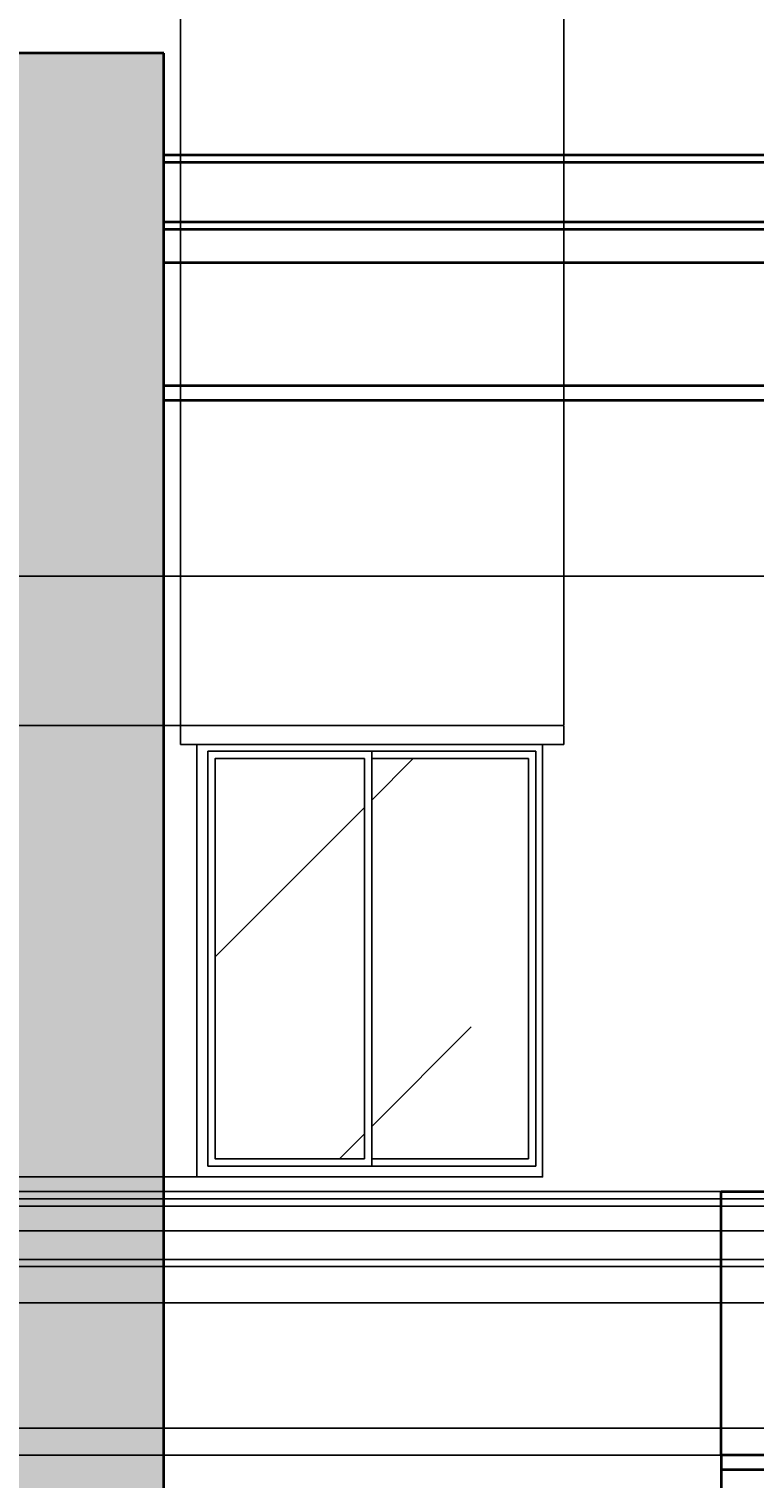
# Model space of a CAD drawing. Units: inches. Extents: x 93 to 565, y 123 to 656.
# Tile 7 of 18: x 192 to 291, y 324 to 522. Entities that reach past the tile are written whole.
import ezdxf

# ---------------------------------------------------------------- set-up
doc = ezdxf.new("R2010")
doc.units = ezdxf.units.IN
doc.header["$MEASUREMENT"] = 0
for name, color, linetype, lineweight in [('A-ANNO-DIMS', 2, 'Continuous', 18), ('A-ELEV', 7, 'Continuous', 35), ('A-GLAZ', 4, 'Continuous', 25), ('A-WALL-PATT', 8, 'Continuous', 13)]:
    doc.layers.add(name, color=color, linetype=linetype, lineweight=lineweight)
doc.styles.get("Standard").update_dxf_attribs({"font": 'arial.ttf'})
doc.dimstyles.get("Standard").update_dxf_attribs({"dimtxt": 0.18, "dimasz": 0.18, "dimexe": 0.18, "dimexo": 0.0625, "dimgap": 0.09, "dimtad": 0, "dimtih": 1, "dimtoh": 1, "dimdec": 4, "dimzin": 0, "dimdsep": 46, "dimtxsty": 'Standard', "dimcen": 0.09, "dimadec": 0, "dimazin": 0, "dimtfac": 1, "dimtdec": 4, "dimtofl": 0, "dimtmove": 0, "dimatfit": 3, "dimfxl": 1, "dimtolj": 1, "dimtzin": 0, "dimarcsym": 0})

# ---------------------------------------------------------------- blocks, each defined once
blk = doc.blocks.new('*U6')
for p, q in [((38.1, 38.1), (38.1, 1476.3)), ((38.1, 1476.3), (607.2, 1476.3)), ((607.2, 38.1), (607.2, 1476.3)), ((607.2, 1476.3), (1176.3, 1476.3)), ((1176.3, 1476.3), (1176.3, 38.1)), ((607.2, 38.1), (38.1, 38.1)), ((1176.3, 38.1), (607.2, 38.1))]:
    blk.add_line(p, q)
blk.add_lwpolyline([(0, 0), (1200, 0), (1200, 1500), (0, 1500)], close=True)
for points in [[(581.8, 1450.9), (581.8, 63.5), (63.5, 63.5), (63.5, 1450.9), (581.8, 1450.9)], [(607.2, 1450.9), (1150.9, 1450.9), (1150.9, 63.5), (607.2, 63.5)]]:
    blk.add_lwpolyline(points)
blk = doc.blocks.new('*D26')
at = {"layer": 'A-ANNO-DIMS', "color": 0, "lineweight": -2, "transparency": 16777216}
for p, q in [((119.08, 519.16), (119.08, 656.13)), ((119.26, 655.95), (328.79, 655.95)), ((538.9, 655.95), (329.37, 655.95)), ((539.08, 630.47), (539.08, 656.13))]:
    blk.add_line(p, q, dxfattribs=at)
at = {"layer": 'A-ANNO-DIMS', "color": 0, "transparency": 16777216}
for points in [[(119.26, 655.98), (119.26, 655.92), (119.08, 655.95)], [(538.9, 655.98), (538.9, 655.92), (539.08, 655.95)]]:
    blk.add_solid(points, dxfattribs=at)
at = {"layer": 'Defpoints', "color": 0, "transparency": 16777216}
for p in [(539.08, 655.95), (539.08, 630.4), (119.08, 519.1)]:
    blk.add_point(p, dxfattribs=at)
at = {"layer": 'A-ANNO-DIMS', "color": 0, "transparency": 16777216, "insert": (329.08, 655.95), "char_height": 0.18, "attachment_point": 5}
blk.add_mtext('\\A1;420', dxfattribs=at)
blk = doc.blocks.new('*D27')
at = {"layer": 'A-ANNO-DIMS', "color": 0, "lineweight": -2, "transparency": 16777216}
for p, q in [((210.54, 519.04), (210.54, 134)), ((119.08, 159.67), (119.08, 134)), ((119.26, 134.18), (164.42, 134.18)), ((210.36, 134.18), (165.21, 134.18))]:
    blk.add_line(p, q, dxfattribs=at)
at = {"layer": 'A-ANNO-DIMS', "color": 0, "transparency": 16777216}
for points in [[(119.26, 134.21), (119.26, 134.15), (119.08, 134.18)], [(210.36, 134.21), (210.36, 134.15), (210.54, 134.18)]]:
    blk.add_solid(points, dxfattribs=at)
at = {"layer": 'Defpoints', "color": 0, "transparency": 16777216}
for p in [(210.54, 519.1), (119.08, 159.73), (210.54, 134.18)]:
    blk.add_point(p, dxfattribs=at)
at = {"layer": 'A-ANNO-DIMS', "color": 0, "transparency": 16777216, "insert": (164.81, 134.18), "char_height": 0.18, "attachment_point": 5}
blk.add_mtext('\\A1;91.46', dxfattribs=at)
blk = doc.blocks.new('*D28')
at = {"layer": 'A-ANNO-DIMS', "color": 0, "lineweight": -2, "transparency": 16777216}
for p, q in [((210.54, 519.04), (210.54, 134)), ((295.69, 183.67), (295.69, 134)), ((210.72, 134.18), (252.72, 134.18)), ((295.51, 134.18), (253.51, 134.18))]:
    blk.add_line(p, q, dxfattribs=at)
at = {"layer": 'A-ANNO-DIMS', "color": 0, "transparency": 16777216}
for points in [[(210.72, 134.21), (210.72, 134.15), (210.54, 134.18)], [(295.51, 134.21), (295.51, 134.15), (295.69, 134.18)]]:
    blk.add_solid(points, dxfattribs=at)
at = {"layer": 'Defpoints', "color": 0, "transparency": 16777216}
for p in [(210.54, 519.1), (295.69, 183.73), (295.69, 134.18)]:
    blk.add_point(p, dxfattribs=at)
at = {"layer": 'A-ANNO-DIMS', "color": 0, "transparency": 16777216, "insert": (253.12, 134.18), "char_height": 0.18, "attachment_point": 5}
blk.add_mtext('\\A1;85.14', dxfattribs=at)
blk = doc.blocks.new('*D31')
at = {"layer": 'A-ANNO-DIMS', "color": 0, "lineweight": -2, "transparency": 16777216}
for p, q in [((417.87, 630.4), (564.81, 630.4)), ((564.63, 630.22), (564.63, 395.25)), ((564.63, 159.91), (564.63, 394.89)), ((119.14, 159.73), (564.81, 159.73))]:
    blk.add_line(p, q, dxfattribs=at)
at = {"layer": 'A-ANNO-DIMS', "color": 0, "transparency": 16777216}
for points in [[(564.6, 630.22), (564.66, 630.22), (564.63, 630.4)], [(564.6, 159.91), (564.66, 159.91), (564.63, 159.73)]]:
    blk.add_solid(points, dxfattribs=at)
at = {"layer": 'Defpoints', "color": 0, "transparency": 16777216}
for p in [(417.81, 630.4), (564.63, 630.4), (119.08, 159.73)]:
    blk.add_point(p, dxfattribs=at)
at = {"layer": 'A-ANNO-DIMS', "color": 0, "transparency": 16777216, "insert": (564.63, 395.07), "char_height": 0.18, "attachment_point": 5}
blk.add_mtext('\\A1;470.7', dxfattribs=at)
blk = doc.blocks.new('*D34')
at = {"layer": 'A-ANNO-DIMS', "color": 0, "lineweight": -2, "transparency": 16777216}
for p, q in [((286.62, 363.73), (93.35, 363.73)), ((93.53, 363.55), (93.53, 338.52)), ((93.53, 313.13), (93.53, 338.16)), ((286.62, 312.95), (93.35, 312.95))]:
    blk.add_line(p, q, dxfattribs=at)
at = {"layer": 'A-ANNO-DIMS', "color": 0, "transparency": 16777216}
for points in [[(93.5, 363.55), (93.56, 363.55), (93.53, 363.73)], [(93.5, 313.13), (93.56, 313.13), (93.53, 312.95)]]:
    blk.add_solid(points, dxfattribs=at)
at = {"layer": 'Defpoints', "color": 0, "transparency": 16777216}
for p in [(93.53, 363.73), (286.69, 363.73), (286.69, 312.95)]:
    blk.add_point(p, dxfattribs=at)
at = {"layer": 'A-ANNO-DIMS', "color": 0, "transparency": 16777216, "insert": (93.53, 338.34), "char_height": 0.18, "attachment_point": 5}
blk.add_mtext('\\A1;50.78', dxfattribs=at)
blk = doc.blocks.new('*D35')
at = {"layer": 'A-ANNO-DIMS', "color": 0, "lineweight": -2, "transparency": 16777216}
for p, q in [((119.02, 519.1), (93.35, 519.1)), ((93.53, 518.92), (93.53, 441.6)), ((93.53, 363.91), (93.53, 441.23)), ((286.62, 363.73), (93.35, 363.73))]:
    blk.add_line(p, q, dxfattribs=at)
at = {"layer": 'A-ANNO-DIMS', "color": 0, "transparency": 16777216}
for points in [[(93.5, 518.92), (93.56, 518.92), (93.53, 519.1)], [(93.5, 363.91), (93.56, 363.91), (93.53, 363.73)]]:
    blk.add_solid(points, dxfattribs=at)
at = {"layer": 'Defpoints', "color": 0, "transparency": 16777216}
for p in [(93.53, 519.1), (119.08, 519.1), (286.69, 363.73)]:
    blk.add_point(p, dxfattribs=at)
at = {"layer": 'A-ANNO-DIMS', "color": 0, "transparency": 16777216, "insert": (93.53, 441.42), "char_height": 0.18, "attachment_point": 5}
blk.add_mtext('\\A1;155.37', dxfattribs=at)
blk = doc.blocks.new('*D36')
at = {"layer": 'A-ANNO-DIMS', "color": 0, "lineweight": -2, "transparency": 16777216}
for p, q in [((417.75, 594.4), (93.35, 594.4)), ((93.53, 594.22), (93.53, 556.93)), ((93.53, 519.28), (93.53, 556.57)), ((119.02, 519.1), (93.35, 519.1))]:
    blk.add_line(p, q, dxfattribs=at)
at = {"layer": 'A-ANNO-DIMS', "color": 0, "transparency": 16777216}
for points in [[(93.5, 594.22), (93.56, 594.22), (93.53, 594.4)], [(93.5, 519.28), (93.56, 519.28), (93.53, 519.1)]]:
    blk.add_solid(points, dxfattribs=at)
at = {"layer": 'Defpoints', "color": 0, "transparency": 16777216}
for p in [(93.53, 594.4), (417.81, 594.4), (119.08, 519.1)]:
    blk.add_point(p, dxfattribs=at)
at = {"layer": 'A-ANNO-DIMS', "color": 0, "transparency": 16777216, "insert": (93.53, 556.75), "char_height": 0.18, "attachment_point": 5}
blk.add_mtext('\\A1;75.3', dxfattribs=at)
blk = doc.blocks.new('*D64')
at = {"layer": 'A-ANNO-DIMS', "color": 0, "lineweight": -2, "transparency": 16777216}
for p, q in [((212.83, 427.41), (212.83, 656.13)), ((213.01, 655.95), (238.63, 655.95)), ((265.03, 655.95), (239.41, 655.95)), ((265.21, 427.41), (265.21, 656.13))]:
    blk.add_line(p, q, dxfattribs=at)
at = {"layer": 'A-ANNO-DIMS', "color": 0, "transparency": 16777216}
for points in [[(213.01, 655.98), (213.01, 655.92), (212.83, 655.95)], [(265.03, 655.98), (265.03, 655.92), (265.21, 655.95)]]:
    blk.add_solid(points, dxfattribs=at)
at = {"layer": 'Defpoints', "color": 0, "transparency": 16777216}
for p in [(265.21, 655.95), (212.83, 427.35), (265.21, 427.35)]:
    blk.add_point(p, dxfattribs=at)
at = {"layer": 'A-ANNO-DIMS', "color": 0, "transparency": 16777216, "insert": (239.02, 655.95), "char_height": 0.18, "attachment_point": 5}
blk.add_mtext('\\A1;52.39', dxfattribs=at)
blk = doc.blocks.new('*D65')
at = {"layer": 'A-ANNO-DIMS', "color": 0, "lineweight": -2, "transparency": 16777216}
for p, q in [((265.15, 427.35), (93.35, 427.35)), ((93.53, 427.17), (93.53, 396.71)), ((93.53, 365.89), (93.53, 396.35)), ((262.24, 365.71), (93.35, 365.71))]:
    blk.add_line(p, q, dxfattribs=at)
at = {"layer": 'A-ANNO-DIMS', "color": 0, "transparency": 16777216}
for points in [[(93.5, 427.17), (93.56, 427.17), (93.53, 427.35)], [(93.5, 365.89), (93.56, 365.89), (93.53, 365.71)]]:
    blk.add_solid(points, dxfattribs=at)
at = {"layer": 'Defpoints', "color": 0, "transparency": 16777216}
for p in [(93.53, 427.35), (265.21, 427.35), (262.3, 365.71)]:
    blk.add_point(p, dxfattribs=at)
at = {"layer": 'A-ANNO-DIMS', "color": 0, "transparency": 16777216, "insert": (93.53, 396.53), "char_height": 0.18, "attachment_point": 5}
blk.add_mtext('\\A1;61.64', dxfattribs=at)
blk = doc.blocks.new('*D72')
at = {"layer": 'A-ANNO-DIMS', "color": 0, "lineweight": -2, "transparency": 16777216}
for p, q in [((295.62, 447.73), (93.35, 447.73)), ((93.53, 447.55), (93.53, 405.91)), ((93.53, 363.91), (93.53, 405.55)), ((286.62, 363.73), (93.35, 363.73))]:
    blk.add_line(p, q, dxfattribs=at)
at = {"layer": 'A-ANNO-DIMS', "color": 0, "transparency": 16777216}
for points in [[(93.5, 447.55), (93.56, 447.55), (93.53, 447.73)], [(93.5, 363.91), (93.56, 363.91), (93.53, 363.73)]]:
    blk.add_solid(points, dxfattribs=at)
at = {"layer": 'Defpoints', "color": 0, "transparency": 16777216}
for p in [(295.69, 447.73), (93.53, 363.73), (286.69, 363.73)]:
    blk.add_point(p, dxfattribs=at)
at = {"layer": 'A-ANNO-DIMS', "color": 0, "transparency": 16777216, "insert": (93.53, 405.73), "char_height": 0.18, "attachment_point": 5}
blk.add_mtext('\\A1;84', dxfattribs=at)
blk = doc.blocks.new('*D105')
at = {"layer": 'A-ANNO-DIMS', "color": 0, "lineweight": -2, "transparency": 16777216}
for p, q in [((119.08, 519.16), (119.08, 656.13)), ((119.26, 655.95), (328.54, 655.95)), ((538.9, 655.95), (329.62, 655.95)), ((539.08, 630.47), (539.08, 656.13))]:
    blk.add_line(p, q, dxfattribs=at)
at = {"layer": 'A-ANNO-DIMS', "color": 0, "transparency": 16777216}
for points in [[(119.26, 655.98), (119.26, 655.92), (119.08, 655.95)], [(538.9, 655.98), (538.9, 655.92), (539.08, 655.95)]]:
    blk.add_solid(points, dxfattribs=at)
at = {"layer": 'Defpoints', "color": 0, "transparency": 16777216}
for p in [(539.08, 655.95), (539.08, 630.4), (119.08, 519.1)]:
    blk.add_point(p, dxfattribs=at)
at = {"layer": 'A-ANNO-DIMS', "color": 0, "transparency": 16777216, "insert": (329.08, 655.95), "char_height": 0.18, "attachment_point": 5}
blk.add_mtext('\\A1;420.000', dxfattribs=at)
blk = doc.blocks.new('*D106')
at = {"layer": 'A-ANNO-DIMS', "color": 0, "lineweight": -2, "transparency": 16777216}
for p, q in [((210.54, 519.04), (210.54, 134)), ((119.08, 159.67), (119.08, 134)), ((119.26, 134.18), (164.35, 134.18)), ((210.36, 134.18), (165.28, 134.18))]:
    blk.add_line(p, q, dxfattribs=at)
at = {"layer": 'A-ANNO-DIMS', "color": 0, "transparency": 16777216}
for points in [[(119.26, 134.21), (119.26, 134.15), (119.08, 134.18)], [(210.36, 134.21), (210.36, 134.15), (210.54, 134.18)]]:
    blk.add_solid(points, dxfattribs=at)
at = {"layer": 'Defpoints', "color": 0, "transparency": 16777216}
for p in [(210.54, 519.1), (119.08, 159.73), (210.54, 134.18)]:
    blk.add_point(p, dxfattribs=at)
at = {"layer": 'A-ANNO-DIMS', "color": 0, "transparency": 16777216, "insert": (164.81, 134.18), "char_height": 0.18, "attachment_point": 5}
blk.add_mtext('\\A1;91.465', dxfattribs=at)
blk = doc.blocks.new('*D107')
at = {"layer": 'A-ANNO-DIMS', "color": 0, "lineweight": -2, "transparency": 16777216}
for p, q in [((210.54, 519.04), (210.54, 134)), ((295.69, 183.67), (295.69, 134)), ((210.72, 134.18), (252.65, 134.18)), ((295.51, 134.18), (253.58, 134.18))]:
    blk.add_line(p, q, dxfattribs=at)
at = {"layer": 'A-ANNO-DIMS', "color": 0, "transparency": 16777216}
for points in [[(210.72, 134.21), (210.72, 134.15), (210.54, 134.18)], [(295.51, 134.21), (295.51, 134.15), (295.69, 134.18)]]:
    blk.add_solid(points, dxfattribs=at)
at = {"layer": 'Defpoints', "color": 0, "transparency": 16777216}
for p in [(210.54, 519.1), (295.69, 183.73), (295.69, 134.18)]:
    blk.add_point(p, dxfattribs=at)
at = {"layer": 'A-ANNO-DIMS', "color": 0, "transparency": 16777216, "insert": (253.12, 134.18), "char_height": 0.18, "attachment_point": 5}
blk.add_mtext('\\A1;85.143', dxfattribs=at)
blk = doc.blocks.new('*D110')
at = {"layer": 'A-ANNO-DIMS', "color": 0, "lineweight": -2, "transparency": 16777216}
for p, q in [((417.87, 630.4), (564.81, 630.4)), ((564.63, 630.22), (564.63, 395.25)), ((564.63, 159.91), (564.63, 394.89)), ((119.14, 159.73), (564.81, 159.73))]:
    blk.add_line(p, q, dxfattribs=at)
at = {"layer": 'A-ANNO-DIMS', "color": 0, "transparency": 16777216}
for points in [[(564.6, 630.22), (564.66, 630.22), (564.63, 630.4)], [(564.6, 159.91), (564.66, 159.91), (564.63, 159.73)]]:
    blk.add_solid(points, dxfattribs=at)
at = {"layer": 'Defpoints', "color": 0, "transparency": 16777216}
for p in [(417.81, 630.4), (564.63, 630.4), (119.08, 159.73)]:
    blk.add_point(p, dxfattribs=at)
at = {"layer": 'A-ANNO-DIMS', "color": 0, "transparency": 16777216, "insert": (564.63, 395.07), "char_height": 0.18, "attachment_point": 5}
blk.add_mtext('\\A1;470.673', dxfattribs=at)
blk = doc.blocks.new('*D113')
at = {"layer": 'A-ANNO-DIMS', "color": 0, "lineweight": -2, "transparency": 16777216}
for p, q in [((286.62, 363.73), (93.35, 363.73)), ((93.53, 363.55), (93.53, 338.52)), ((93.53, 313.13), (93.53, 338.16)), ((286.62, 312.95), (93.35, 312.95))]:
    blk.add_line(p, q, dxfattribs=at)
at = {"layer": 'A-ANNO-DIMS', "color": 0, "transparency": 16777216}
for points in [[(93.5, 363.55), (93.56, 363.55), (93.53, 363.73)], [(93.5, 313.13), (93.56, 313.13), (93.53, 312.95)]]:
    blk.add_solid(points, dxfattribs=at)
at = {"layer": 'Defpoints', "color": 0, "transparency": 16777216}
for p in [(93.53, 363.73), (286.69, 363.73), (286.69, 312.95)]:
    blk.add_point(p, dxfattribs=at)
at = {"layer": 'A-ANNO-DIMS', "color": 0, "transparency": 16777216, "insert": (93.53, 338.34), "char_height": 0.18, "attachment_point": 5}
blk.add_mtext('\\A1;50.783', dxfattribs=at)
blk = doc.blocks.new('*D114')
at = {"layer": 'A-ANNO-DIMS', "color": 0, "lineweight": -2, "transparency": 16777216}
for p, q in [((119.02, 519.1), (93.35, 519.1)), ((93.53, 518.92), (93.53, 441.6)), ((93.53, 363.91), (93.53, 441.23)), ((286.62, 363.73), (93.35, 363.73))]:
    blk.add_line(p, q, dxfattribs=at)
at = {"layer": 'A-ANNO-DIMS', "color": 0, "transparency": 16777216}
for points in [[(93.5, 518.92), (93.56, 518.92), (93.53, 519.1)], [(93.5, 363.91), (93.56, 363.91), (93.53, 363.73)]]:
    blk.add_solid(points, dxfattribs=at)
at = {"layer": 'Defpoints', "color": 0, "transparency": 16777216}
for p in [(93.53, 519.1), (119.08, 519.1), (286.69, 363.73)]:
    blk.add_point(p, dxfattribs=at)
at = {"layer": 'A-ANNO-DIMS', "color": 0, "transparency": 16777216, "insert": (93.53, 441.42), "char_height": 0.18, "attachment_point": 5}
blk.add_mtext('\\A1;155.368', dxfattribs=at)
blk = doc.blocks.new('*D115')
at = {"layer": 'A-ANNO-DIMS', "color": 0, "lineweight": -2, "transparency": 16777216}
for p, q in [((417.75, 594.4), (93.35, 594.4)), ((93.53, 594.22), (93.53, 556.93)), ((93.53, 519.28), (93.53, 556.57)), ((119.02, 519.1), (93.35, 519.1))]:
    blk.add_line(p, q, dxfattribs=at)
at = {"layer": 'A-ANNO-DIMS', "color": 0, "transparency": 16777216}
for points in [[(93.5, 594.22), (93.56, 594.22), (93.53, 594.4)], [(93.5, 519.28), (93.56, 519.28), (93.53, 519.1)]]:
    blk.add_solid(points, dxfattribs=at)
at = {"layer": 'Defpoints', "color": 0, "transparency": 16777216}
for p in [(93.53, 594.4), (417.81, 594.4), (119.08, 519.1)]:
    blk.add_point(p, dxfattribs=at)
at = {"layer": 'A-ANNO-DIMS', "color": 0, "transparency": 16777216, "insert": (93.53, 556.75), "char_height": 0.18, "attachment_point": 5}
blk.add_mtext('\\A1;75.305', dxfattribs=at)
blk = doc.blocks.new('*D143')
at = {"layer": 'A-ANNO-DIMS', "color": 0, "lineweight": -2, "transparency": 16777216}
for p, q in [((212.83, 427.41), (212.83, 656.13)), ((213.01, 655.95), (238.56, 655.95)), ((265.03, 655.95), (239.48, 655.95)), ((265.21, 427.41), (265.21, 656.13))]:
    blk.add_line(p, q, dxfattribs=at)
at = {"layer": 'A-ANNO-DIMS', "color": 0, "transparency": 16777216}
for points in [[(213.01, 655.98), (213.01, 655.92), (212.83, 655.95)], [(265.03, 655.98), (265.03, 655.92), (265.21, 655.95)]]:
    blk.add_solid(points, dxfattribs=at)
at = {"layer": 'Defpoints', "color": 0, "transparency": 16777216}
for p in [(265.21, 655.95), (212.83, 427.35), (265.21, 427.35)]:
    blk.add_point(p, dxfattribs=at)
at = {"layer": 'A-ANNO-DIMS', "color": 0, "transparency": 16777216, "insert": (239.02, 655.95), "char_height": 0.18, "attachment_point": 5}
blk.add_mtext('\\A1;52.388', dxfattribs=at)
blk = doc.blocks.new('*D144')
at = {"layer": 'A-ANNO-DIMS', "color": 0, "lineweight": -2, "transparency": 16777216}
for p, q in [((265.15, 427.35), (93.35, 427.35)), ((93.53, 427.17), (93.53, 396.71)), ((93.53, 365.89), (93.53, 396.35)), ((262.24, 365.71), (93.35, 365.71))]:
    blk.add_line(p, q, dxfattribs=at)
at = {"layer": 'A-ANNO-DIMS', "color": 0, "transparency": 16777216}
for points in [[(93.5, 427.17), (93.56, 427.17), (93.53, 427.35)], [(93.5, 365.89), (93.56, 365.89), (93.53, 365.71)]]:
    blk.add_solid(points, dxfattribs=at)
at = {"layer": 'Defpoints', "color": 0, "transparency": 16777216}
for p in [(93.53, 427.35), (265.21, 427.35), (262.3, 365.71)]:
    blk.add_point(p, dxfattribs=at)
at = {"layer": 'A-ANNO-DIMS', "color": 0, "transparency": 16777216, "insert": (93.53, 396.53), "char_height": 0.18, "attachment_point": 5}
blk.add_mtext('\\A1;61.638', dxfattribs=at)
blk = doc.blocks.new('*D151')
at = {"layer": 'A-ANNO-DIMS', "color": 0, "lineweight": -2, "transparency": 16777216}
for p, q in [((295.62, 447.73), (93.35, 447.73)), ((93.53, 447.55), (93.53, 405.91)), ((93.53, 363.91), (93.53, 405.55)), ((286.62, 363.73), (93.35, 363.73))]:
    blk.add_line(p, q, dxfattribs=at)
at = {"layer": 'A-ANNO-DIMS', "color": 0, "transparency": 16777216}
for points in [[(93.5, 447.55), (93.56, 447.55), (93.53, 447.73)], [(93.5, 363.91), (93.56, 363.91), (93.53, 363.73)]]:
    blk.add_solid(points, dxfattribs=at)
at = {"layer": 'Defpoints', "color": 0, "transparency": 16777216}
for p in [(295.69, 447.73), (93.53, 363.73), (286.69, 363.73)]:
    blk.add_point(p, dxfattribs=at)
at = {"layer": 'A-ANNO-DIMS', "color": 0, "transparency": 16777216, "insert": (93.53, 405.73), "char_height": 0.18, "attachment_point": 5}
blk.add_mtext('\\A1;84.000', dxfattribs=at)
blk = doc.blocks.new('*D190')
at = {"layer": 'A-ANNO-DIMS', "color": 0, "lineweight": -2, "transparency": 16777216}
for p, q in [((514.58, 348.55), (93.35, 348.55)), ((93.53, 348.37), (93.53, 338.33)), ((93.53, 327.91), (93.53, 337.96)), ((539.02, 327.73), (93.35, 327.73))]:
    blk.add_line(p, q, dxfattribs=at)
at = {"layer": 'A-ANNO-DIMS', "color": 0, "transparency": 16777216}
for points in [[(93.5, 348.37), (93.56, 348.37), (93.53, 348.55)], [(93.5, 327.91), (93.56, 327.91), (93.53, 327.73)]]:
    blk.add_solid(points, dxfattribs=at)
at = {"layer": 'Defpoints', "color": 0, "transparency": 16777216}
for p in [(93.53, 348.55), (514.64, 348.55), (539.08, 327.73)]:
    blk.add_point(p, dxfattribs=at)
at = {"layer": 'A-ANNO-DIMS', "color": 0, "transparency": 16777216, "insert": (93.53, 338.14), "char_height": 0.18, "attachment_point": 5}
blk.add_mtext('\\A1;20.822', dxfattribs=at)
blk = doc.blocks.new('*D191')
at = {"layer": 'A-ANNO-DIMS', "color": 0, "lineweight": -2, "transparency": 16777216}
for p, q in [((514.58, 353.47), (93.35, 353.47)), ((93.53, 353.29), (93.53, 351.2)), ((93.53, 348.73), (93.53, 350.83)), ((514.58, 348.55), (93.35, 348.55))]:
    blk.add_line(p, q, dxfattribs=at)
at = {"layer": 'A-ANNO-DIMS', "color": 0, "transparency": 16777216}
for points in [[(93.5, 353.29), (93.56, 353.29), (93.53, 353.47)], [(93.5, 348.73), (93.56, 348.73), (93.53, 348.55)]]:
    blk.add_solid(points, dxfattribs=at)
at = {"layer": 'Defpoints', "color": 0, "transparency": 16777216}
for p in [(93.53, 353.47), (514.64, 353.47), (514.64, 348.55)]:
    blk.add_point(p, dxfattribs=at)
at = {"layer": 'A-ANNO-DIMS', "color": 0, "transparency": 16777216, "insert": (93.53, 351.01), "char_height": 0.18, "attachment_point": 5}
blk.add_mtext('\\A1;4.918', dxfattribs=at)
blk = doc.blocks.new('*D192')
at = {"layer": 'A-ANNO-DIMS', "color": 0, "lineweight": -2, "transparency": 16777216}
for p, q in [((514.58, 354.47), (93.35, 354.47)), ((514.58, 353.47), (93.35, 353.47)), ((93.53, 354.29), (93.53, 354.15)), ((93.53, 353.65), (93.53, 353.79))]:
    blk.add_line(p, q, dxfattribs=at)
at = {"layer": 'A-ANNO-DIMS', "color": 0, "transparency": 16777216}
for points in [[(93.5, 354.29), (93.56, 354.29), (93.53, 354.47)], [(93.5, 353.65), (93.56, 353.65), (93.53, 353.47)]]:
    blk.add_solid(points, dxfattribs=at)
at = {"layer": 'Defpoints', "color": 0, "transparency": 16777216}
for p in [(93.53, 354.47), (514.64, 354.47), (514.64, 353.47)]:
    blk.add_point(p, dxfattribs=at)
at = {"layer": 'A-ANNO-DIMS', "color": 0, "transparency": 16777216, "insert": (93.53, 353.97), "char_height": 0.18, "attachment_point": 5}
blk.add_mtext('\\A1;1.000', dxfattribs=at)
blk = doc.blocks.new('*D193')
at = {"layer": 'A-ANNO-DIMS', "color": 0, "lineweight": -2, "transparency": 16777216}
for p, q in [((514.58, 358.37), (93.35, 358.37)), ((93.53, 358.19), (93.53, 356.61)), ((514.58, 354.47), (93.35, 354.47)), ((93.53, 354.65), (93.53, 356.24))]:
    blk.add_line(p, q, dxfattribs=at)
at = {"layer": 'A-ANNO-DIMS', "color": 0, "transparency": 16777216}
for points in [[(93.5, 358.19), (93.56, 358.19), (93.53, 358.37)], [(93.5, 354.65), (93.56, 354.65), (93.53, 354.47)]]:
    blk.add_solid(points, dxfattribs=at)
at = {"layer": 'Defpoints', "color": 0, "transparency": 16777216}
for p in [(93.53, 358.37), (514.64, 358.37), (514.64, 354.47)]:
    blk.add_point(p, dxfattribs=at)
at = {"layer": 'A-ANNO-DIMS', "color": 0, "transparency": 16777216, "insert": (93.53, 356.42), "char_height": 0.18, "attachment_point": 5}
blk.add_mtext('\\A1;3.901', dxfattribs=at)
blk = doc.blocks.new('*D194')
at = {"layer": 'A-ANNO-DIMS', "color": 0, "lineweight": -2, "transparency": 16777216}
for p, q in [((524.92, 361.75), (93.35, 361.75)), ((93.53, 361.57), (93.53, 360.24)), ((514.58, 358.37), (93.35, 358.37)), ((93.53, 358.55), (93.53, 359.88))]:
    blk.add_line(p, q, dxfattribs=at)
at = {"layer": 'A-ANNO-DIMS', "color": 0, "transparency": 16777216}
for points in [[(93.5, 361.57), (93.56, 361.57), (93.53, 361.75)], [(93.5, 358.55), (93.56, 358.55), (93.53, 358.37)]]:
    blk.add_solid(points, dxfattribs=at)
at = {"layer": 'Defpoints', "color": 0, "transparency": 16777216}
for p in [(93.53, 361.75), (524.99, 361.75), (514.64, 358.37)]:
    blk.add_point(p, dxfattribs=at)
at = {"layer": 'A-ANNO-DIMS', "color": 0, "transparency": 16777216, "insert": (93.53, 360.06), "char_height": 0.18, "attachment_point": 5}
blk.add_mtext('\\A1;3.374', dxfattribs=at)
blk = doc.blocks.new('*D195')
at = {"layer": 'A-ANNO-DIMS', "color": 0, "lineweight": -2, "transparency": 16777216}
for p, q in [((524.92, 362.75), (93.35, 362.75)), ((93.53, 362.57), (93.53, 362.43)), ((524.92, 361.75), (93.35, 361.75)), ((93.53, 361.93), (93.53, 362.07))]:
    blk.add_line(p, q, dxfattribs=at)
at = {"layer": 'A-ANNO-DIMS', "color": 0, "transparency": 16777216}
for points in [[(93.5, 362.57), (93.56, 362.57), (93.53, 362.75)], [(93.5, 361.93), (93.56, 361.93), (93.53, 361.75)]]:
    blk.add_solid(points, dxfattribs=at)
at = {"layer": 'Defpoints', "color": 0, "transparency": 16777216}
for p in [(93.53, 362.75), (524.99, 362.75), (524.99, 361.75)]:
    blk.add_point(p, dxfattribs=at)
at = {"layer": 'A-ANNO-DIMS', "color": 0, "transparency": 16777216, "insert": (93.53, 362.25), "char_height": 0.18, "attachment_point": 5}
blk.add_mtext('\\A1;1.000', dxfattribs=at)
blk = doc.blocks.new('*D196')
at = {"layer": 'A-ANNO-DIMS', "color": 0, "lineweight": -2, "transparency": 16777216}
for p, q in [((524.92, 363.73), (93.35, 363.73)), ((524.92, 362.75), (93.35, 362.75)), ((93.53, 363.55), (93.53, 363.42)), ((93.53, 362.93), (93.53, 363.06))]:
    blk.add_line(p, q, dxfattribs=at)
at = {"layer": 'A-ANNO-DIMS', "color": 0, "transparency": 16777216}
for points in [[(93.5, 363.55), (93.56, 363.55), (93.53, 363.73)], [(93.5, 362.93), (93.56, 362.93), (93.53, 362.75)]]:
    blk.add_solid(points, dxfattribs=at)
at = {"layer": 'Defpoints', "color": 0, "transparency": 16777216}
for p in [(93.53, 363.73), (524.99, 363.73), (524.99, 362.75)]:
    blk.add_point(p, dxfattribs=at)
at = {"layer": 'A-ANNO-DIMS', "color": 0, "transparency": 16777216, "insert": (93.53, 363.24), "char_height": 0.18, "attachment_point": 5}
blk.add_mtext('\\A1;0.985', dxfattribs=at)
blk = doc.blocks.new('*D198')
at = {"layer": 'A-ANNO-DIMS', "color": 0, "lineweight": -2, "transparency": 16777216}
for p, q in [((515.95, 331.43), (93.35, 331.43)), ((93.53, 331.25), (93.53, 329.76)), ((93.53, 327.91), (93.53, 329.4)), ((539.02, 327.73), (93.35, 327.73))]:
    blk.add_line(p, q, dxfattribs=at)
at = {"layer": 'A-ANNO-DIMS', "color": 0, "transparency": 16777216}
for points in [[(93.5, 331.25), (93.56, 331.25), (93.53, 331.43)], [(93.5, 327.91), (93.56, 327.91), (93.53, 327.73)]]:
    blk.add_solid(points, dxfattribs=at)
at = {"layer": 'Defpoints', "color": 0, "transparency": 16777216}
for p in [(93.53, 331.43), (516.01, 331.43), (539.08, 327.73)]:
    blk.add_point(p, dxfattribs=at)
at = {"layer": 'A-ANNO-DIMS', "color": 0, "transparency": 16777216, "insert": (93.53, 329.58), "char_height": 0.18, "attachment_point": 5}
blk.add_mtext('\\A1;3.701', dxfattribs=at)

msp = doc.modelspace()

# ---------------------------------------------------------------- hatches: boundary and pattern name
at = {"layer": 'A-GLAZ'}
h = msp.add_hatch(dxfattribs=at)
h.set_pattern_fill('GOST_GLASS', color=256, scale=21)
h.set_pattern_definition([(45, (0, 0), (178.19, 0), [105, -147]), (45, (44.55, 0), (178.19, 0), [42, -210]), (45, (0, 44.55), (178.19, 0), [42, -210])])
h.paths.add_polyline_path([(237.9617, 422.832), (217.5562, 422.832), (217.5562, 368.21), (237.9617, 368.21)])
h.paths.add_polyline_path([(260.3673, 422.832), (238.9617, 422.832), (238.9617, 368.21), (260.3673, 368.21)])
at = {"layer": 'A-WALL-PATT'}
h = msp.add_hatch(dxfattribs=at)
h.set_pattern_fill('STARS', color=256, scale=21)
h.paths.add_polyline_path([(210.5443, 507.7323), (210.5443, 519.0999), (119.0794, 519.0999), (119.0794, 507.7323), (119.0794, 183.7323), (210.5443, 183.7323)])
h.paths.add_polyline_path([(187.648, 430.1508), (187.648, 391.4653), (143.2118, 391.4653), (143.2118, 430.1508)], flags=16)
h.paths.add_polyline_path([(187.648, 455.6579), (143.2118, 455.6579), (143.2118, 494.3434), (187.648, 494.3434)], flags=16)
h.paths.add_polyline_path([(184.648, 427.1508), (184.648, 394.4653), (146.2118, 394.4653), (146.2118, 427.1508)], flags=0)
h.paths.add_polyline_path([(184.648, 458.6579), (146.2118, 458.6579), (146.2118, 491.3434), (184.648, 491.3434)], flags=0)
h.paths.add_polyline_path([(187.648, 363.1705), (187.648, 324.485), (143.2118, 324.485), (143.2118, 363.1705)], flags=16)
h.paths.add_polyline_path([(184.648, 360.1705), (184.648, 327.485), (146.2118, 327.485), (146.2118, 360.1705)], flags=0)
h.paths.add_polyline_path([(187.648, 300.3249), (187.648, 261.6394), (143.2118, 261.6394), (143.2118, 300.3249)], flags=16)
h.paths.add_polyline_path([(184.648, 297.3249), (184.648, 264.6394), (146.2118, 264.6394), (146.2118, 297.3249)], flags=0)
h.paths.add_polyline_path([(187.648, 243.6441), (187.648, 204.9587), (143.2118, 204.9587), (143.2118, 243.6441)], flags=16)
h.paths.add_polyline_path([(184.648, 240.6441), (184.648, 207.9587), (146.2118, 207.9587), (146.2118, 240.6441)], flags=0)

# ---------------------------------------------------------------- linework, layer by layer
at = {"layer": 'A-ELEV'}
for p, q in [((210.5443, 519.0999), (119.0794, 519.0999)), ((210.5443, 507.7323), (210.5443, 519.0999)), ((210.5443, 183.7323), (210.5443, 507.7323)), ((399.6946, 505.2018), (210.5443, 505.2018)), ((399.6946, 504.2018), (210.5443, 504.2018)), ((375.0121, 496.0418), (210.5443, 496.0418)), ((375.0121, 495.0418), (210.5443, 495.0418)), ((375.0121, 490.4746), (210.5443, 490.4746)), ((210.5443, 473.7323), (437.1885, 473.7323)), ((210.5443, 471.7323), (437.1885, 471.7323)), ((286.6874, 327.7323), (286.6874, 363.7323)), ((286.6874, 363.7323), (295.6874, 363.7323)), ((295.6874, 327.7323), (286.6874, 327.7323)), ((286.6874, 327.7323), (286.6874, 312.9491)), ((295.6874, 325.7323), (286.6874, 325.7323))]:
    msp.add_line(p, q, dxfattribs=at)
at = {"layer": 'A-GLAZ'}
for p, q in [((265.2145, 427.3478), (212.8266, 427.3478)), ((212.8266, 427.3478), (212.8266, 424.7651)), ((265.2145, 424.7651), (265.2145, 427.3478)), ((212.8266, 424.7651), (216.5562, 424.7651)), ((262.3003, 424.7651), (265.2145, 424.7651))]:
    msp.add_line(p, q, dxfattribs=at)

# ---------------------------------------------------------------- block references
at = {"layer": 'A-GLAZ', "xscale": 0.0393700787401575, "yscale": 0.0393700787401575, "zscale": 0.0393700787401575}
msp.add_blockref('*U6', (215.0562, 365.71), dxfattribs=at)

# ---------------------------------------------------------------- dimensions: what is measured, and where the dimension line sits
at = {"layer": 'A-ANNO-DIMS'}
for base, p1, p2, override, picture, middle in [((539.0794, 655.9548), (119.0794, 519.0999), (539.0794, 630.4048), {"dimdec": 0, "dimlfac": 1, "dimrnd": 0, "dimzin": 0, "dimdsep": 46, "dimlunit": 2}, '*D26', (329.0794, 655.9548)), ((539.0794, 655.9548), (119.0794, 519.0999), (539.0794, 630.4048), {"dimdec": 3, "dimlfac": 1, "dimrnd": 0, "dimzin": 0, "dimdsep": 46, "dimlunit": 2}, '*D105', (329.0794, 655.9548)), ((265.2145, 655.9548), (212.8266, 427.3478), (265.2145, 427.3478), {"dimdec": 2, "dimlfac": 1, "dimrnd": 0, "dimzin": 0, "dimdsep": 46, "dimlunit": 2}, '*D64', (239.0206, 655.9548)), ((265.2145, 655.9548), (212.8266, 427.3478), (265.2145, 427.3478), {"dimdec": 3, "dimlfac": 1, "dimrnd": 0, "dimzin": 0, "dimdsep": 46, "dimlunit": 2}, '*D143', (239.0206, 655.9548)), ((210.5443, 134.1823), (119.0794, 159.7323), (210.5443, 519.0999), {"dimdec": 2, "dimlfac": 1, "dimrnd": 0, "dimzin": 0, "dimdsep": 46, "dimlunit": 2}, '*D27', (164.8118, 134.1823)), ((210.5443, 134.1823), (119.0794, 159.7323), (210.5443, 519.0999), {"dimdec": 3, "dimlfac": 1, "dimrnd": 0, "dimzin": 0, "dimdsep": 46, "dimlunit": 2}, '*D106', (164.8118, 134.1823)), ((295.6874, 134.1823), (210.5443, 519.0999), (295.6874, 183.7323), {"dimdec": 2, "dimlfac": 1, "dimrnd": 0, "dimzin": 0, "dimdsep": 46, "dimlunit": 2}, '*D28', (253.1158, 134.1823)), ((295.6874, 134.1823), (210.5443, 519.0999), (295.6874, 183.7323), {"dimdec": 3, "dimlfac": 1, "dimrnd": 0, "dimzin": 0, "dimdsep": 46, "dimlunit": 2}, '*D107', (253.1158, 134.1823))]:
    dim = msp.add_linear_dim(base=base, p1=p1, p2=p2, dimstyle='Standard', override=override, dxfattribs=at)
    dim.commit()
    dim.dimension.update_dxf_attribs({"geometry": picture, "text_midpoint": middle})
for base, p1, p2, override, picture, middle in [((564.6294, 630.4048), (119.0794, 159.7323), (417.8097, 630.4048), {"dimdec": 1, "dimlfac": 1, "dimrnd": 0, "dimzin": 0, "dimdsep": 46, "dimlunit": 2}, '*D31', (564.6294, 395.0685)), ((564.62936, 630.40478), (119.07936, 159.73225), (417.80971, 630.40477), {"dimdec": 3, "dimlfac": 1, "dimrnd": 0, "dimzin": 0, "dimdsep": 46, "dimlunit": 2}, '*D110', (564.62936, 395.06851)), ((93.5294, 594.4048), (119.0794, 519.0999), (417.8097, 594.4048), {"dimdec": 3, "dimlfac": 1, "dimrnd": 0, "dimzin": 0, "dimdsep": 46, "dimlunit": 2}, '*D115', (93.5294, 556.7523)), ((93.5294, 594.4048), (119.0794, 519.0999), (417.8097, 594.4048), {"dimdec": 1, "dimlfac": 1, "dimrnd": 0, "dimzin": 0, "dimdsep": 46, "dimlunit": 2}, '*D36', (93.5294, 556.7523)), ((93.5294, 519.0999), (286.6874, 363.7323), (119.0794, 519.0999), {"dimdec": 3, "dimlfac": 1, "dimrnd": 0, "dimzin": 0, "dimdsep": 46, "dimlunit": 2}, '*D114', (93.5294, 441.4161)), ((93.5294, 519.0999), (286.6874, 363.7323), (119.0794, 519.0999), {"dimdec": 2, "dimlfac": 1, "dimrnd": 0, "dimzin": 0, "dimdsep": 46, "dimlunit": 2}, '*D35', (93.5294, 441.4161)), ((93.5294, 363.7323), (295.6874, 447.7323), (286.6874, 363.7323), {"dimdec": 3, "dimlfac": 1, "dimrnd": 0, "dimzin": 0, "dimdsep": 46, "dimlunit": 2}, '*D151', (93.5294, 405.7323)), ((93.5294, 363.7323), (295.6874, 447.7323), (286.6874, 363.7323), {"dimdec": 0, "dimlfac": 1, "dimrnd": 0, "dimzin": 0, "dimdsep": 46, "dimlunit": 2}, '*D72', (93.5294, 405.7323)), ((93.5294, 427.3478), (262.3003, 365.71), (265.2145, 427.3478), {"dimdec": 3, "dimlfac": 1, "dimrnd": 0, "dimzin": 0, "dimdsep": 46, "dimlunit": 2}, '*D144', (93.5294, 396.5289)), ((93.5294, 427.3478), (262.3003, 365.71), (265.2145, 427.3478), {"dimdec": 2, "dimlfac": 1, "dimrnd": 0, "dimzin": 0, "dimdsep": 46, "dimlunit": 2}, '*D65', (93.5294, 396.5289)), ((93.5294, 363.7323), (286.6874, 312.9491), (286.6874, 363.7323), {"dimdec": 3, "dimlfac": 1, "dimrnd": 0, "dimzin": 0, "dimdsep": 46, "dimlunit": 2}, '*D113', (93.5294, 338.3407)), ((93.5294, 363.7323), (286.6874, 312.9491), (286.6874, 363.7323), {"dimdec": 2, "dimlfac": 1, "dimrnd": 0, "dimzin": 0, "dimdsep": 46, "dimlunit": 2}, '*D34', (93.5294, 338.3407)), ((93.5294, 363.7323), (524.9864, 362.7477), (524.9864, 363.7323), {"dimdec": 3, "dimlfac": 1, "dimrnd": 0, "dimzin": 0, "dimdsep": 46, "dimlunit": 2}, '*D196', (93.5294, 363.24)), ((93.5294, 362.7477), (524.9864, 361.7477), (524.9864, 362.7477), {"dimdec": 3, "dimlfac": 1, "dimrnd": 0, "dimzin": 0, "dimdsep": 46, "dimlunit": 2}, '*D195', (93.5294, 362.2477)), ((93.5294, 361.7477), (514.6424, 358.3735), (524.9864, 361.7477), {"dimdec": 3, "dimlfac": 1, "dimrnd": 0, "dimzin": 0, "dimdsep": 46, "dimlunit": 2}, '*D194', (93.5294, 360.0606)), ((93.5294, 358.3735), (514.6424, 354.4729), (514.6424, 358.3735), {"dimdec": 3, "dimlfac": 1, "dimrnd": 0, "dimzin": 0, "dimdsep": 46, "dimlunit": 2}, '*D193', (93.5294, 356.4232)), ((93.5294, 354.4729), (514.6424, 353.4729), (514.6424, 354.4729), {"dimdec": 3, "dimlfac": 1, "dimrnd": 0, "dimzin": 0, "dimdsep": 46, "dimlunit": 2}, '*D192', (93.5294, 353.9729)), ((93.5294, 353.4729), (514.6424, 348.5546), (514.6424, 353.4729), {"dimdec": 3, "dimlfac": 1, "dimrnd": 0, "dimzin": 0, "dimdsep": 46, "dimlunit": 2}, '*D191', (93.5294, 351.0137)), ((93.5294, 348.5546), (539.0794, 327.7323), (514.6424, 348.5546), {"dimdec": 3, "dimlfac": 1, "dimrnd": 0, "dimzin": 0, "dimdsep": 46, "dimlunit": 2}, '*D190', (93.5294, 338.1434)), ((93.5294, 331.4335), (539.0794, 327.7323), (516.0099, 331.4335), {"dimdec": 3, "dimlfac": 1, "dimrnd": 0, "dimzin": 0, "dimdsep": 46, "dimlunit": 2}, '*D198', (93.5294, 329.5829))]:
    dim = msp.add_linear_dim(base=base, p1=p1, p2=p2, angle=90, dimstyle='Standard', override=override, dxfattribs=at)
    dim.commit()
    dim.dimension.update_dxf_attribs({"geometry": picture, "text_midpoint": middle})

doc.saveas('drawing.dxf')
